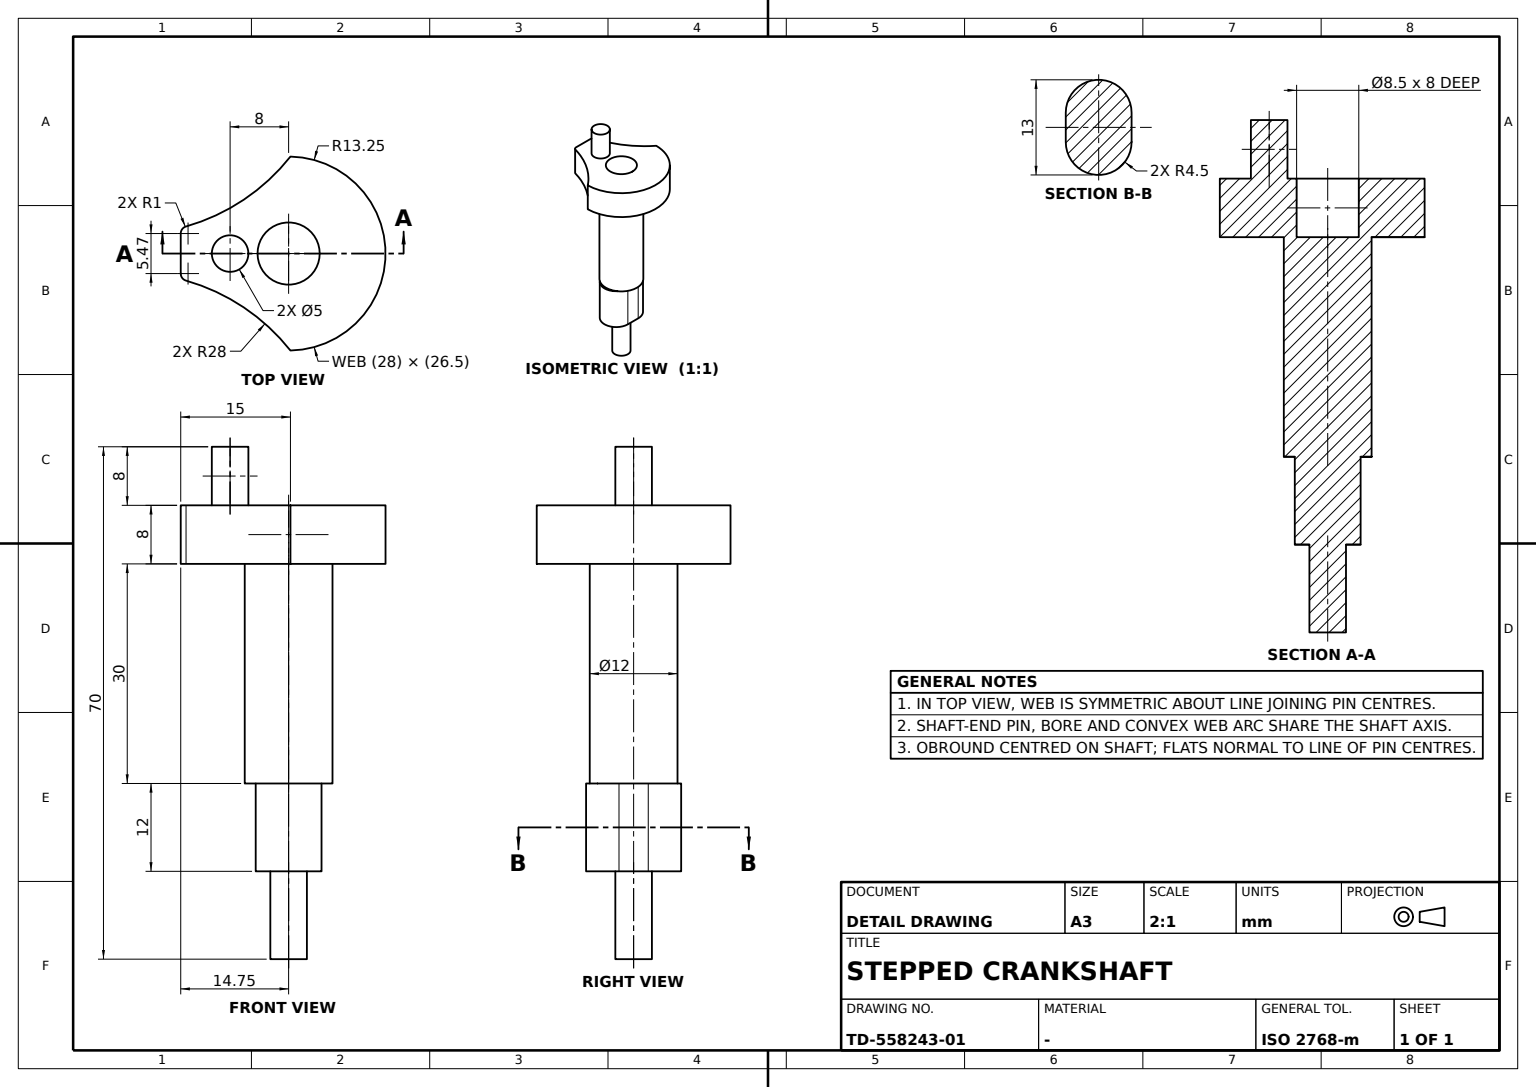
CATIA V5 part; units mm, degrees
sketch "Sketch1" plane through (0, 0, 0) normal (0, 0, 1) x (0, 1, 0)
  point P0 (-3.5, 0)
  line L0 (-3.5, 0) -> (3.5, 0)
  arc A0 (3.5, 0) -> (13.2476, -15) centre (30.6218, 6.9577) ccw
  point P1 (13.2476, -15)
  point P2 (-13.2476, -15)
  arc A1 (-13.2476, -15) -> (-3.5, 0) centre (-30.6218, 6.9577) ccw
  circle A2 centre (0, -14.75) radius 4.25
  point P3 (0, -14.75)
  point P4 (0, -21)
  arc A3 (-13.2476, -15) -> (13.2476, -15) centre (0, -14.75) ccw
  dimension "radius A0" = 28
  dimension "length L0" = 7
  dimension "radius A2" = 4.25
  dimension "radius A3" = 13.25
  dimension "distance P2 x axis" = 15
  dimension "distance x axis A3" = 28
  constraint coincidence P0 x-axis
  constraint coincidence P3 y-axis
  constraint horizontal L0 x-axis
  constraint symmetry P2 P1 y-axis
  constraint symmetry A1 A0 y-axis
  constraint concentricity A2 A3
extrude "Pad1" add sketch "Sketch1" along normal blind 8
fillet "Fillet1" radius 1 2 edges at (0, -3.5, 4) (0, 3.5, 4)
sketch "Sketch2" plane through (0, 0, 8) normal (0, 0, 1) x (1, 0, 0)
  circle A0 centre (6.75, 0) radius 2.5
  point P0 (6.75, 0)
  circle A1 centre (14.75, 0) radius 4.25 construction
  dimension "radius A0" = 2.5
  dimension "distance A0 A1" = 1.25
  constraint coincidence P0 x-axis
extrude "Pad2" add sketch "Sketch2" along normal blind 8
sketch "Sketch3" plane through (0, 0, 0) normal (0, 0, -1) x (1, 0, 0)
  circle A0 centre (14.75, 0) radius 6
  point P0 (14.75, 0)
  circle A1 centre (14.75, 0) radius 4.25 construction
  dimension "radius A0" = 6
  constraint coincidence P0 x-axis
  constraint concentricity A0 A1
extrude "Pad3" add sketch "Sketch3" along normal blind 30
sketch "Sketch4" plane through (0, 0, -30) normal (0, 0, -1) x (1, 0, 0)
  line L0 (14.75, 2) -> (14.75, -2) construction
  line L1 (19.25, 2) -> (19.25, -2)
  line L2 (10.25, -2) -> (10.25, 2)
  arc A0 (19.25, -2) -> (10.25, -2) centre (14.75, -2) cw
  arc A1 (10.25, 2) -> (19.25, 2) centre (14.75, 2) cw
  arc A2 (15, -13.2476) -> (15, 13.2476) centre (14.75, 0) ccw construction
  dimension "distance L0 L1" = 4.5
  dimension "distance A1 A0" = 13
  dimension "distance L0 A2" = 13.25
  constraint vertical L0 y-axis
  constraint tangency A0 L1
  constraint tangency A1 L1
  constraint tangency A0 L2
  constraint tangency A1 L2
  constraint symmetry A0 A1 x-axis
extrude "Pad4" add sketch "Sketch4" along normal blind 12
sketch "Sketch5" plane through (0, 0, -42) normal (0, 0, -1) x (0, 1, 0)
  circle A0 centre (0, 14.75) radius 2.5
  point P0 (0, 14.75)
  circle A1 centre (0, 14.75) radius 6 construction
  dimension "radius A0" = 2.5
  constraint coincidence P0 y-axis
  constraint concentricity A0 A1
extrude "Pad5" add sketch "Sketch5" along normal blind 12
